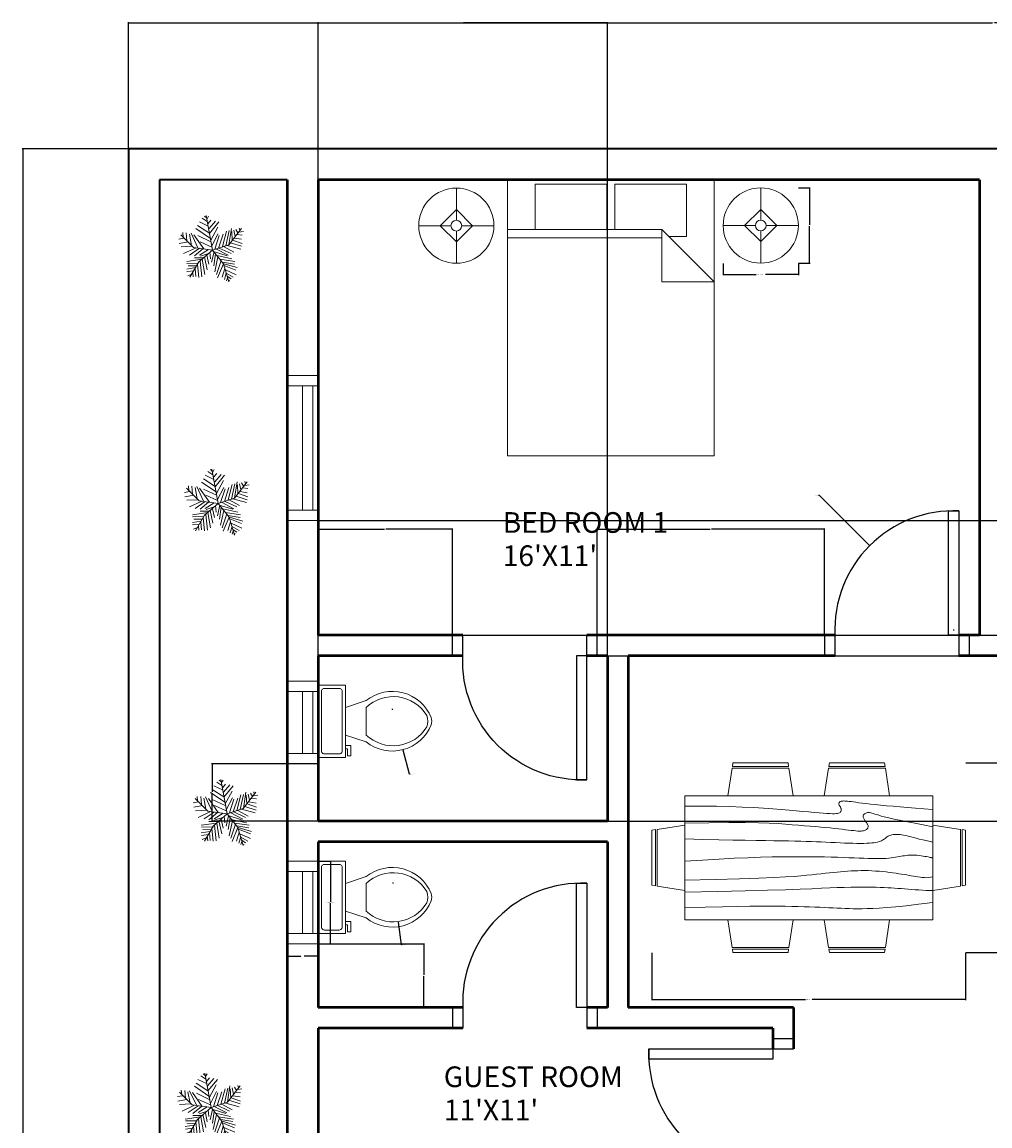
# Model space of a CAD drawing. Units: inches. Extents: x 156 to 720, y 11 to 679.
# Tile 4 of 5: x 156 to 437, y 359 to 679. Entities that reach past the tile are written whole.
import ezdxf

# ---------------------------------------------------------------- set-up
doc = ezdxf.new("R2010")
doc.units = ezdxf.units.IN
for name, color, linetype, lineweight in [('A-ANNO-DIMS', 2, 'Continuous', 18), ('A-AREA-IDEN', 7, 'Continuous', 25), ('A-DOOR', 3, 'Continuous', 25), ('A-FLOR-FIXT', 9, 'Continuous', 18), ('A-FURN', 8, 'Continuous', 18), ('A-GLAZ', 4, 'Continuous', 18), ('A-WALL', 7, 'Continuous', 50), ('C-PROP', 7, 'Continuous', 35), ('E-LITE', 2, 'Continuous', 13), ('L-PLNT', 94, 'Continuous', 13)]:
    doc.layers.add(name, color=color, linetype=linetype, lineweight=lineweight)
doc.styles.get("Standard").update_dxf_attribs({"font": 'arial.ttf'})
doc.dimstyles.get("Standard").update_dxf_attribs({"dimtxt": 0.18, "dimasz": 0.18, "dimexe": 0.18, "dimexo": 0.0625, "dimgap": 0.09, "dimtad": 0, "dimtih": 1, "dimtoh": 1, "dimdec": 4, "dimzin": 0, "dimdsep": 46, "dimtxsty": 'Standard', "dimcen": 0.09, "dimadec": 0, "dimazin": 0, "dimtfac": 1, "dimtdec": 4, "dimtofl": 0, "dimtmove": 0, "dimatfit": 3, "dimfxl": 1, "dimtolj": 1, "dimtzin": 0, "dimarcsym": 0})

# ---------------------------------------------------------------- blocks, each defined once
blk = doc.blocks.new('Bed - Queen')
for p, q in [((0, -80.00003), (0, 0)), ((0, 0), (59.99999, 0)), ((59.99999, 0), (59.99999, -80.00003)), ((7.99999, -1.2), (28.79998, -1.2)), ((7.99999, -14.4), (7.99999, -1.2)), ((28.79998, -1.2), (28.79998, -14.4)), ((31.19999, -1.2), (51.99999, -1.2)), ((31.19999, -14.4), (31.19999, -1.2)), ((51.99999, -1.2), (51.99999, -16.4)), ((0, -14.4), (44.8, -14.4)), ((59.99999, -29.6), (44.8, -14.4)), ((44.8, -14.4), (44.8, -29.6)), ((44.8, -16.8), (0, -16.8)), ((51.99999, -16.4), (46.79936, -16.4)), ((44.8, -29.6), (59.99999, -29.6)), ((59.99999, -80.00003), (0, -80.00003))]:
    blk.add_line(p, q)
blk = doc.blocks.new('Lamp - Table')
for p, q in [((0, 7), (0, 1)), ((0, 3), (-3, 0)), ((3, 0), (0, 3)), ((-1, 0), (-7, 0)), ((-3, 0), (0, -3)), ((0, -3), (3, 0)), ((1, 0), (7, 0)), ((0, -1), (0, -7))]:
    blk.add_line(p, q)
for radius in [7, 1]:
    blk.add_circle((0, 0), radius)
blk = doc.blocks.new('Toilet - top')
for p, q in [((9.5, -6), (9.5, -2)), ((-10, -8.5), (-8, -8.5)), ((-10, -9.5), (-10, -8.5)), ((-7, -9.5), (-10, -9.5)), ((-8, -8.5), (-8, -8)), ((-7, -8), (-7, -9.5)), ((-4, -8), (-6, -14)), ((4, -8), (6, -14)), ((4, -14), (-4, -14))]:
    blk.add_line(p, q)
blk.add_lwpolyline([(10.5, -8), (10.5, 0), (-10.5, 0), (-10.5, -8)], close=True)
for points in [[(-9.5, -2), (-9.5, -6)], [(8.5, -1), (-8.5, -1)], [(-8.5, -7), (8.5, -7)]]:
    blk.add_lwpolyline(points)
for centre, radius, start, end in [((-8.62, -1.88), 0.884, 81.8699, 188.1301), ((8.62, -1.88), 0.884, 351.8699, 98.1301), ((-8.62, -6.12), 0.884, 171.8699, 278.1301), ((8.62, -6.12), 0.884, 261.8699, 8.1301), ((3.52, -21.58), 12.17, 141.4691, 247.9714), ((4.2, -21.82), 11.33, 136.3677, 238.9468), ((-3.52, -21.58), 12.17, 292.0284, 38.5307), ((-4.2, -21.82), 11.33, 301.053, 43.6321), ((0, -27.88), 4, 245.7318, 294.2682), ((0, -29), 4, 254.8605, 285.1395)]:
    blk.add_arc(centre, radius, start, end)
blk = doc.blocks.new('Dining Set - 36 x 72 in.')
for p, q in [((-22.2343, 26.00059), (-23.4847, 17.99762)), ((-22.2304, 26), (-5.7608, 26)), ((-22, 27.5), (-22.1562, 26.50042)), ((-5.8416, 26.5), (-22.1534, 26.5)), ((-22, 27.5), (-6, 27.5)), ((-5.8437, 26.49966), (-6, 27.5)), ((-4.5152, 17.99762), (-5.7655, 25.99926)), ((5.7657, 26.00059), (4.5153, 17.99762)), ((5.7696, 26), (22.2392, 26)), ((6, 27.5), (5.8438, 26.50042)), ((22.1584, 26.5), (5.8466, 26.5)), ((6, 27.5), (22, 27.5)), ((22.1563, 26.49966), (22, 27.5)), ((23.4848, 17.99762), (22.2345, 25.99926)), ((36, 18), (-36, 18)), ((-36, 18), (-36, -18)), ((36, -18), (36, 18)), ((-45.5, 8), (-44.5004, 8.15617)), ((-45.5, 8), (-45.5, -8)), ((-44.5, -8.15843), (-44.5, 8.15338)), ((-44.0006, 8.23428), (-35.9976, 9.48474)), ((-44, 8.23041), (-44, -8.23915)), ((44.0006, 8.23428), (35.9976, 9.48474)), ((44, 8.23041), (44, -8.23915)), ((44.5, -8.15843), (44.5, 8.15338)), ((45.5, 8), (44.5005, 8.15617)), ((45.5, 8), (45.5, -8)), ((-44.4997, -8.15631), (-45.5, -8)), ((-35.9976, -9.48476), (-43.9993, -8.2345)), ((35.9976, -9.48476), (43.9993, -8.2345)), ((44.4997, -8.15631), (45.5, -8)), ((-36, -18), (36, -18)), ((-22.2343, -26.0006), (-23.4847, -17.99762)), ((-4.5152, -17.99762), (-5.7655, -25.99928)), ((5.7657, -26.0006), (4.5153, -17.99762)), ((23.4848, -17.99762), (22.2345, -25.99928)), ((-22.2304, -26), (-5.7608, -26)), ((-22, -27.5), (-22.1562, -26.50044)), ((-5.8416, -26.5), (-22.1534, -26.5)), ((-22, -27.5), (-6, -27.5)), ((-5.8437, -26.49967), (-6, -27.5)), ((5.7696, -26), (22.2392, -26)), ((6, -27.5), (5.8438, -26.50044)), ((22.1584, -26.5), (5.8466, -26.5)), ((6, -27.5), (22, -27.5)), ((22.1563, -26.49967), (22, -27.5))]:
    blk.add_line(p, q)
for points in [[(-36, 15), (-31.1772, 14.97754), (-26.8079, 14.91406), (-22.8538, 14.81543), (-19.276, 14.6875), (-16.0362, 14.53613), (-13.0957, 14.36718), (-10.4159, 14.18652), (-7.9583, 14), (-5.6904, 13.81315), (-3.6035, 13.63021), (-1.6954, 13.45508), (0.0365, 13.29166), (1.5945, 13.14388), (2.9811, 13.01562), (4.1988, 12.9108), (5.25, 12.83333), (6.1393, 12.78613), (6.8802, 12.76823), (7.4883, 12.77767), (7.9792, 12.8125), (8.3685, 12.87077), (8.6719, 12.95052), (8.9049, 13.0498), (9.0833, 13.16666), (9.2205, 13.29899), (9.3216, 13.44401), (9.3895, 13.59879), (9.4271, 13.76041), (9.4373, 13.92594), (9.4232, 14.09245), (9.3875, 14.257), (9.3333, 14.41666), (9.2638, 14.56917), (9.1836, 14.71484), (9.0975, 14.85465), (9.0104, 14.98958), (8.9272, 15.1206), (8.8529, 15.2487), (8.7922, 15.37483), (8.75, 15.5), (8.7305, 15.62467), (8.7344, 15.74739), (8.7617, 15.86621), (8.8125, 15.97916), (8.8867, 16.08431), (8.9844, 16.17968), (9.1055, 16.26334), (9.25, 16.33333), (9.4189, 16.38802), (9.6172, 16.42708), (9.8506, 16.45052), (10.125, 16.45833), (10.4463, 16.45052), (10.8203, 16.42708), (11.2529, 16.38802), (11.75, 16.33333), (12.3184, 16.26318), (12.9694, 16.17838), (13.7151, 16.07991), (14.5677, 15.96875), (15.5395, 15.84586), (16.6426, 15.71224), (17.8893, 15.56884), (19.2917, 15.41666), (20.859, 15.25667), (22.5879, 15.08984), (24.4721, 14.91715), (26.5052, 14.73958), (28.6809, 14.5581), (30.9929, 14.3737), (33.4347, 14.18733), (36, 14)], [(-36, 10), (-28.9766, 10.14274), (-23.1725, 10.20442), (-18.4241, 10.19775), (-14.5677, 10.13541), (-11.4399, 10.03011), (-8.877, 9.89453), (-6.7154, 9.74137), (-4.7917, 9.58333), (-2.9698, 9.43082), (-1.2246, 9.28515), (0.4415, 9.14534), (2.026, 9.01041), (3.5266, 8.87939), (4.9408, 8.7513), (6.266, 8.62516), (7.5, 8.5), (8.6411, 8.37549), (9.6914, 8.2539), (10.6538, 8.13818), (11.5312, 8.03125), (12.3267, 7.93603), (13.043, 7.85547), (13.6831, 7.79248), (14.25, 7.75), (14.7471, 7.7303), (15.1797, 7.73307), (15.5537, 7.75732), (15.875, 7.80208), (16.1494, 7.86637), (16.3828, 7.94922), (16.5811, 8.04964), (16.75, 8.16666), (16.8944, 8.29915), (17.0143, 8.44531), (17.1089, 8.60319), (17.1771, 8.77083), (17.218, 8.94629), (17.2305, 9.1276), (17.2137, 9.31282), (17.1667, 9.5), (17.0895, 9.6875), (16.987, 9.875), (16.8649, 10.0625), (16.7292, 10.25), (16.5856, 10.4375), (16.4401, 10.625), (16.2985, 10.8125), (16.1667, 11), (16.05, 11.18733), (15.9518, 11.3737), (15.8752, 11.5581), (15.8229, 11.73958), (15.798, 11.91715), (15.8034, 12.08984), (15.842, 12.25667), (15.9167, 12.41666), (16.0295, 12.56836), (16.1784, 12.70833), (16.3605, 12.83268), (16.5729, 12.9375), (16.8127, 13.01888), (17.0768, 13.07291), (17.3625, 13.0957), (17.6667, 13.08333), (17.9894, 13.03312), (18.3418, 12.94726), (18.7382, 12.82918), (19.1927, 12.68229), (19.7195, 12.51001), (20.3327, 12.31575), (21.0465, 12.10294), (21.875, 11.875), (22.8357, 11.63354), (23.959, 11.37304), (25.2786, 11.08618), (26.8282, 10.76562), (28.6414, 10.40405), (30.752, 9.99414), (33.1936, 9.52856), (36, 9)], [(-36, 5.5), (-30.7157, 5.3348), (-26.069, 5.20963), (-21.9946, 5.11767), (-18.4271, 5.05208), (-15.3009, 5.00602), (-12.5508, 4.97265), (-10.1112, 4.94515), (-7.9167, 4.91666), (-5.909, 4.88167), (-4.0586, 4.83984), (-2.3429, 4.79215), (-0.7396, 4.73958), (0.7739, 4.6831), (2.22, 4.6237), (3.6213, 4.56233), (5, 4.5), (6.373, 4.43782), (7.7344, 4.3776), (9.0723, 4.32129), (10.375, 4.27083), (11.6309, 4.22819), (12.8281, 4.19531), (13.9551, 4.17415), (15, 4.16666), (15.954, 4.17448), (16.819, 4.19791), (17.6001, 4.23698), (18.3021, 4.29166), (18.9299, 4.36198), (19.4883, 4.44791), (19.9823, 4.54948), (20.4167, 4.66666), (20.7969, 4.79899), (21.1302, 4.94401), (21.4245, 5.09879), (21.6875, 5.26041), (21.9271, 5.42594), (22.1511, 5.59245), (22.3672, 5.757), (22.5834, 5.91666), (22.8065, 6.06868), (23.0404, 6.21093), (23.2879, 6.34147), (23.5521, 6.45833), (23.8358, 6.55957), (24.142, 6.64323), (24.4735, 6.70735), (24.8334, 6.75), (25.2235, 6.76969), (25.642, 6.76692), (26.0858, 6.74267), (26.5521, 6.69791), (27.0379, 6.63362), (27.5404, 6.55078), (28.0565, 6.45036), (28.5834, 6.33333), (29.1242, 6.19987), (29.7071, 6.04687), (30.3661, 5.87044), (31.1354, 5.66666), (32.0493, 5.43164), (33.142, 5.16146), (34.4475, 4.85221), (36, 4.5)], [(-36, -1), (-30.7915, -0.6591), (-26.0195, -0.38216), (-21.6519, -0.16284), (-17.6563, 0.00521), (-14.0005, 0.12833), (-10.6523, 0.21289), (-7.5796, 0.26522), (-4.75, 0.29166), (-2.134, 0.29793), (0.2878, 0.28711), (2.5317, 0.26163), (4.6146, 0.22396), (6.5529, 0.17651), (8.3633, 0.12174), (10.0623, 0.06209), (11.6667, 0), (13.1899, -0.06201), (14.6341, -0.1211), (15.9982, -0.17432), (17.2813, -0.21875), (18.4823, -0.25147), (19.6003, -0.26953), (20.6343, -0.27002), (21.5834, -0.25), (22.4481, -0.20768), (23.2357, -0.14584), (23.9549, -0.06836), (24.6146, 0.02083), (25.2235, 0.11784), (25.7904, 0.21875), (26.3241, 0.31966), (26.8334, 0.41666), (27.3265, 0.50618), (27.8099, 0.58593), (28.2894, 0.65397), (28.7709, 0.70833), (29.2601, 0.74707), (29.763, 0.76823), (30.2855, 0.76985), (30.8334, 0.75), (31.4088, 0.70784), (31.9994, 0.64713), (32.589, 0.57275), (33.1615, 0.48958), (33.7008, 0.4025), (34.1908, 0.3164), (34.6153, 0.23616), (34.9584, 0.16666), (35.2099, 0.11165), (35.3848, 0.07031), (35.504, 0.04069), (35.5886, 0.02083), (35.6594, 0.00879), (35.7377, 0.0026), (35.8442, 0.00032), (36, 0)], [(-36, -6.5), (-27.1843, -6.31267), (-20.084, -6.1263), (-14.469, -5.9419), (-10.1094, -5.76042), (-6.7752, -5.58285), (-4.2363, -5.41016), (-2.2629, -5.24333), (-0.625, -5.08334), (0.8708, -4.93099), (2.2715, -4.78646), (3.5872, -4.64974), (4.8281, -4.52084), (6.0046, -4.39974), (7.127, -4.28646), (8.2053, -4.18099), (9.25, -4.08334), (10.2705, -3.99382), (11.2734, -3.91407), (12.2647, -3.84603), (13.25, -3.79167), (14.2354, -3.75293), (15.2266, -3.73177), (16.2295, -3.73015), (17.25, -3.75), (18.2912, -3.79248), (19.3451, -3.85547), (20.4009, -3.93604), (21.4479, -4.03125), (22.4754, -4.13819), (23.4727, -4.25391), (24.4289, -4.37549), (25.3334, -4.5), (26.1785, -4.62492), (26.9694, -4.74935), (27.7145, -4.87281), (28.4219, -4.99479), (29.1, -5.11483), (29.7572, -5.23242), (30.4016, -5.34709), (31.0417, -5.45834), (31.6837, -5.56437), (32.3262, -5.65821), (32.9658, -5.73153), (33.599, -5.77604), (34.2224, -5.78345), (34.8327, -5.74545), (35.4264, -5.65373), (36, -5.5)], [(-36, -10), (-26.4022, -9.81299), (-18.4675, -9.62891), (-11.9839, -9.45069), (-6.7396, -9.28125), (-2.5226, -9.12354), (0.8789, -8.98047), (3.6769, -8.85498), (6.0833, -8.75), (8.2767, -8.66765), (10.3021, -8.60677), (12.1712, -8.56543), (13.8958, -8.54167), (15.4876, -8.53353), (16.9583, -8.53907), (18.3197, -8.55632), (19.5834, -8.58334), (20.7616, -8.61841), (21.8685, -8.66081), (22.9188, -8.71004), (23.9271, -8.76563), (24.9081, -8.82707), (25.8763, -8.89388), (26.8465, -8.96558), (27.8334, -9.04167), (28.8474, -9.12118), (29.8828, -9.20117), (30.93, -9.27824), (31.9792, -9.34896), (33.0205, -9.40991), (34.0443, -9.45768), (35.0407, -9.48885), (36, -9.5)], [(-36, -14.5), (-30.0881, -14.33513), (-25.0332, -14.21224), (-20.7312, -14.12647), (-17.0781, -14.07292), (-13.97, -14.04671), (-11.3027, -14.04297), (-8.9724, -14.05681), (-6.875, -14.08334), (-4.9224, -14.11833), (-3.0905, -14.16016), (-1.3709, -14.20785), (0.2448, -14.26042), (1.7647, -14.3169), (3.1973, -14.3763), (4.5507, -14.43767), (5.8333, -14.5), (7.0554, -14.5621), (8.235, -14.62175), (9.3922, -14.67652), (10.5469, -14.72396), (11.7192, -14.76164), (12.929, -14.78711), (14.1965, -14.79794), (15.5417, -14.79167), (16.9933, -14.76424), (18.6152, -14.70508), (20.4804, -14.60197), (22.6615, -14.44271), (25.2312, -14.21509), (28.2624, -13.9069), (31.8277, -13.50594), (36, -13)]]:
    blk.add_lwpolyline(points)
blk = doc.blocks.new('*U13')
for p, q in [((-10.186, 53.64), (-13.084, 55.962)), ((0, 0), (-10.5, 57)), ((-9.099, 51.782), (-6.563, 55.962)), ((-5.114, 28.097), (-24.676, 40.636)), ((-7.288, 39.707), (-21.778, 46.673)), ((-8.737, 47.138), (-17.069, 52.711)), ((-7.65, 43.423), (-2.578, 49.46)), ((-5.839, 35.992), (4.667, 48.067)), ((-5.114, 27.632), (10.463, 46.673)), ((-2.941, 16.486), (8.652, 37.85)), ((-47.498, 19.737), (-55.83, 18.344)), ((-31.5, 4.5), (-52.5, 25.5)), ((-48.585, 21.131), (-49.309, 29.026)), ((-43.513, 28.561), (-42.427, 15.558)), ((-38.442, 26.239), (-34.819, 7.663)), ((-35.544, 28.097), (-24.314, 3.947)), ((-14.533, 2.09), (-30.834, 25.31)), ((-3.665, 19.273), (-27.574, 35.527)), ((-24.314, 23.917), (-2.941, 13.7)), ((-1.129, 6.734), (9.014, 26.704)), ((3.942, 1.625), (11.187, 24.381)), ((10.101, 3.483), (17.708, 26.239)), ((16.259, 5.805), (23.142, 31.348)), ((22.055, 7.198), (27.489, 32.277)), ((27, 9), (48, 36)), ((27.127, 9.056), (31.112, 35.992)), ((31.836, 30.883), (32.561, 16.486)), ((35.096, 32.741), (37.27, 22.524)), ((36.183, 19.737), (48.137, 17.88)), ((38.719, 34.134), (41.979, 28.561)), ((40.53, 25.775), (48.862, 24.846)), ((43.791, 29.954), (51.036, 30.883)), ((44.153, 36.456), (45.239, 32.741)), ((-40.615, 13.7), (-55.105, 10.913)), ((-33.37, 6.269), (-52.207, 5.34)), ((-28.299, 3.483), (-47.86, -5.805)), ((-21.416, 3.018), (-38.079, -8.128)), ((0, 0), (-31.5, 4.5)), ((-15.982, 2.09), (-30.11, -9.521)), ((0, 0), (-22.5, -19.5)), ((-6.563, 1.161), (-21.416, -8.128)), ((-20.691, 13.7), (-1.129, 4.876)), ((0, 0), (27, 9)), ((0, 0), (18, -22.5)), ((6.478, 1.625), (26.04, -8.592)), ((11.187, 3.483), (30.749, -5.805)), ((18.07, 5.805), (35.096, -3.483)), ((24.229, 7.663), (46.688, 1.625)), ((29.662, 12.307), (48.137, 6.269)), ((33.285, 16.486), (48.862, 10.913)), ((-17.431, -15.094), (-42.789, -18.809)), ((-15.257, -12.772), (-30.11, -12.772)), ((-6.563, -5.805), (-19.967, -9.985)), ((-17.069, -15.094), (-12.721, -40.172)), ((-13.446, -11.378), (-8.737, -32.741)), ((-9.461, -8.592), (-6.201, -23.453)), ((-4.752, -3.483), (-3.665, -14.629)), ((2.493, -3.019), (-1.491, -20.202)), ((1.769, -2.555), (24.229, -9.521)), ((5.029, -6.27), (2.131, -25.775)), ((9.014, -11.378), (3.58, -35.992)), ((14.085, -16.951), (6.478, -40.172)), ((7.565, -9.056), (32.198, -14.629)), ((12.274, -15.094), (36.907, -18.809)), ((-28.299, -29.026), (-42.789, -31.348)), ((-24.314, -21.596), (-42.427, -22.06)), ((-30.834, -34.135), (-42.427, -35.528)), ((-26.849, -26.24), (-40.253, -25.775)), ((-22.5, -19.5), (-37.5, -45)), ((-29.023, -30.884), (-27.936, -43.887)), ((-25.038, -23.918), (-22.865, -45.281)), ((-20.691, -18.345), (-17.793, -44.352)), ((18.07, -22.524), (8.289, -45.745)), ((20.244, -30.419), (15.897, -44.816)), ((16.259, -19.738), (36.183, -22.989)), ((18, -22.5), (27, -52.5)), ((18.433, -22.524), (40.53, -29.026)), ((19.157, -25.311), (38.719, -33.206)), ((21.331, -32.741), (39.081, -40.636)), ((-34.457, -39.708), (-40.978, -42.494)), ((-32.646, -36.921), (-31.921, -44.352)), ((22.78, -37.85), (19.519, -48.532)), ((22.78, -38.314), (34.372, -44.816)), ((24.591, -45.745), (23.142, -50.854)), ((24.591, -43.423), (30.749, -47.603)), ((26.764, -49.925), (28.213, -50.854))]:
    blk.add_line(p, q)
blk = doc.blocks.new('DOOR-SWING-36IN')
for p, q in [((0, 6), (0, 0)), ((3, 6), (3, 0)), ((39, 6), (39, 0)), ((42, 6), (42, 0))]:
    blk.add_line(p, q)
blk.add_lwpolyline([(39, 6), (36, 6), (36, 42), (39, 42)], close=True)
blk.add_arc((37.5, 7.5), 34.53, 87.5104, 182.4896)
blk = doc.blocks.new('WIN-36IN-WALL9')
for p, q in [((0, 9), (0, 0)), ((39, 9), (3, 9)), ((3, 9), (3, 0)), ((3, 7.5), (39, 7.5)), ((39, 0), (39, 9)), ((42, 0), (42, 9)), ((3, 4.5), (39, 4.5)), ((3, 0), (39, 0))]:
    blk.add_line(p, q)
blk = doc.blocks.new('WIN-18IN-WALL9')
for p, q in [((9, 24), (0, 24)), ((0, 21), (0, 3)), ((9, 21), (0, 21)), ((4.5, 21), (4.5, 3)), ((7.5, 21), (7.5, 3)), ((9, 3), (9, 21)), ((0, 3), (9, 3)), ((0, 0), (9, 0))]:
    blk.add_line(p, q)
blk = doc.blocks.new('*D23')
at = {"layer": 'A-ANNO-DIMS', "color": 0, "lineweight": -2, "transparency": 16777216}
for p, q in [((359.29, 608.96), (359.29, 605.57)), ((381.12, 608.96), (381.12, 605.57)), ((359.47, 605.75), (368.87, 605.75)), ((380.94, 605.75), (371.55, 605.75))]:
    blk.add_line(p, q, dxfattribs=at)
at = {"layer": 'A-ANNO-DIMS', "color": 0, "transparency": 16777216}
for points in [[(359.47, 605.78), (359.47, 605.72), (359.29, 605.75)], [(380.94, 605.78), (380.94, 605.72), (381.12, 605.75)]]:
    blk.add_solid(points, dxfattribs=at)
at = {"layer": 'Defpoints', "color": 0, "transparency": 16777216}
for p in [(359.29, 609.02), (381.12, 609.02), (381.12, 605.75)]:
    blk.add_point(p, dxfattribs=at)
at = {"layer": 'A-ANNO-DIMS', "color": 0, "transparency": 16777216, "insert": (370.21, 605.75), "char_height": 0.18, "attachment_point": 5}
blk.add_mtext('\\A1;TABLE LAMP 22 TYP.', dxfattribs=at)
blk = doc.blocks.new('*D24')
at = {"layer": 'A-ANNO-DIMS', "color": 0, "lineweight": -2, "transparency": 16777216}
for p, q in [((381.18, 630.84), (384.57, 630.84)), ((384.39, 630.66), (384.39, 620.11)), ((384.39, 609.2), (384.39, 619.75)), ((381.18, 609.02), (384.57, 609.02))]:
    blk.add_line(p, q, dxfattribs=at)
at = {"layer": 'A-ANNO-DIMS', "color": 0, "transparency": 16777216}
for points in [[(384.36, 630.66), (384.42, 630.66), (384.39, 630.84)], [(384.36, 609.2), (384.42, 609.2), (384.39, 609.02)]]:
    blk.add_solid(points, dxfattribs=at)
at = {"layer": 'Defpoints', "color": 0, "transparency": 16777216}
for p in [(381.12, 630.84), (384.39, 630.84), (381.12, 609.02)]:
    blk.add_point(p, dxfattribs=at)
at = {"layer": 'A-ANNO-DIMS', "color": 0, "transparency": 16777216, "insert": (384.39, 619.93), "char_height": 0.18, "attachment_point": 5}
blk.add_mtext('\\A1;22 TYP.', dxfattribs=at)
blk = doc.blocks.new('*D31')
at = {"layer": 'A-ANNO-DIMS', "color": 0, "lineweight": -2, "transparency": 16777216}
for p, q in [((241.79, 435.59), (245.5, 435.59)), ((245.32, 435.41), (245.32, 423.77)), ((245.32, 411.77), (245.32, 423.41)), ((241.79, 411.59), (245.5, 411.59))]:
    blk.add_line(p, q, dxfattribs=at)
at = {"layer": 'A-ANNO-DIMS', "color": 0, "transparency": 16777216}
for points in [[(245.29, 435.41), (245.35, 435.41), (245.32, 435.59)], [(245.29, 411.77), (245.35, 411.77), (245.32, 411.59)]]:
    blk.add_solid(points, dxfattribs=at)
at = {"layer": 'Defpoints', "color": 0, "transparency": 16777216}
for p in [(241.72, 435.59), (245.32, 435.59), (241.72, 411.59)]:
    blk.add_point(p, dxfattribs=at)
at = {"layer": 'A-ANNO-DIMS', "color": 0, "transparency": 16777216, "insert": (245.32, 423.59), "char_height": 0.18, "attachment_point": 5}
blk.add_mtext('\\A1;WINDOW B 24 TYP.', dxfattribs=at)
blk = doc.blocks.new('*D32')
at = {"layer": 'A-ANNO-DIMS', "color": 0, "lineweight": -2, "transparency": 16777216}
for p, q in [((232.72, 411.53), (232.72, 407.81)), ((241.72, 411.53), (241.72, 407.81)), ((232.9, 407.99), (236.77, 407.99)), ((241.54, 407.99), (237.68, 407.99))]:
    blk.add_line(p, q, dxfattribs=at)
at = {"layer": 'A-ANNO-DIMS', "color": 0, "transparency": 16777216}
for points in [[(232.9, 408.02), (232.9, 407.96), (232.72, 407.99)], [(241.54, 408.02), (241.54, 407.96), (241.72, 407.99)]]:
    blk.add_solid(points, dxfattribs=at)
at = {"layer": 'Defpoints', "color": 0, "transparency": 16777216}
for p in [(232.72, 411.59), (241.72, 411.59), (241.72, 407.99)]:
    blk.add_point(p, dxfattribs=at)
at = {"layer": 'A-ANNO-DIMS', "color": 0, "transparency": 16777216, "insert": (237.22, 407.99), "char_height": 0.18, "attachment_point": 5}
blk.add_mtext('\\A1;9 TYP.', dxfattribs=at)
blk = doc.blocks.new('*D41')
at = {"layer": 'A-ANNO-DIMS', "color": 0, "lineweight": -2, "transparency": 16777216}
for p, q in [((338.64, 408.99), (338.64, 395.23)), ((429.64, 408.99), (429.64, 395.23)), ((338.82, 395.41), (383.18, 395.41)), ((429.46, 395.41), (385.09, 395.41))]:
    blk.add_line(p, q, dxfattribs=at)
at = {"layer": 'A-ANNO-DIMS', "color": 0, "transparency": 16777216}
for points in [[(338.82, 395.44), (338.82, 395.38), (338.64, 395.41)], [(429.46, 395.44), (429.46, 395.38), (429.64, 395.41)]]:
    blk.add_solid(points, dxfattribs=at)
at = {"layer": 'Defpoints', "color": 0, "transparency": 16777216}
for p in [(338.64, 409.06), (429.64, 409.06), (429.64, 395.41)]:
    blk.add_point(p, dxfattribs=at)
at = {"layer": 'A-ANNO-DIMS', "color": 0, "transparency": 16777216, "insert": (384.14, 395.41), "char_height": 0.18, "attachment_point": 5}
blk.add_mtext('\\A1;DINING SET 91', dxfattribs=at)
blk = doc.blocks.new('*D42')
at = {"layer": 'A-ANNO-DIMS', "color": 0, "lineweight": -2, "transparency": 16777216}
for p, q in [((429.7, 464.06), (443.47, 464.06)), ((443.29, 463.88), (443.29, 436.74)), ((443.29, 409.24), (443.29, 436.37)), ((429.7, 409.06), (443.47, 409.06))]:
    blk.add_line(p, q, dxfattribs=at)
at = {"layer": 'A-ANNO-DIMS', "color": 0, "transparency": 16777216}
for points in [[(443.26, 463.88), (443.32, 463.88), (443.29, 464.06)], [(443.26, 409.24), (443.32, 409.24), (443.29, 409.06)]]:
    blk.add_solid(points, dxfattribs=at)
at = {"layer": 'Defpoints', "color": 0, "transparency": 16777216}
for p in [(429.64, 464.06), (443.29, 464.06), (429.64, 409.06)]:
    blk.add_point(p, dxfattribs=at)
at = {"layer": 'A-ANNO-DIMS', "color": 0, "transparency": 16777216, "insert": (443.29, 436.56), "char_height": 0.18, "attachment_point": 5}
blk.add_mtext('\\A1;55', dxfattribs=at)
blk = doc.blocks.new('*D49')
at = {"layer": 'A-ANNO-DIMS', "color": 0, "lineweight": -2, "transparency": 16777216}
for p, q in [((186.72, 642.21), (186.72, 678.94)), ((688.72, 642.21), (688.72, 678.94)), ((186.9, 678.76), (437.44, 678.76)), ((688.54, 678.76), (438.01, 678.76))]:
    blk.add_line(p, q, dxfattribs=at)
at = {"layer": 'A-ANNO-DIMS', "color": 0, "transparency": 16777216}
for points in [[(186.9, 678.79), (186.9, 678.73), (186.72, 678.76)], [(688.54, 678.79), (688.54, 678.73), (688.72, 678.76)]]:
    blk.add_solid(points, dxfattribs=at)
at = {"layer": 'Defpoints', "color": 0, "transparency": 16777216}
for p in [(688.72, 678.76), (186.72, 642.15), (688.72, 642.15)]:
    blk.add_point(p, dxfattribs=at)
at = {"layer": 'A-ANNO-DIMS', "color": 0, "transparency": 16777216, "insert": (437.72, 678.76), "char_height": 0.18, "attachment_point": 5}
blk.add_mtext('\\A1;502', dxfattribs=at)
blk = doc.blocks.new('*D50')
at = {"layer": 'A-ANNO-DIMS', "color": 0, "lineweight": -2, "transparency": 16777216}
for p, q in [((186.66, 642.15), (155.84, 642.15)), ((156.02, 641.97), (156.02, 342.33)), ((156.02, 42.33), (156.02, 341.97)), ((186.66, 42.15), (155.84, 42.15))]:
    blk.add_line(p, q, dxfattribs=at)
at = {"layer": 'A-ANNO-DIMS', "color": 0, "transparency": 16777216}
for points in [[(155.99, 641.97), (156.05, 641.97), (156.02, 642.15)], [(155.99, 42.33), (156.05, 42.33), (156.02, 42.15)]]:
    blk.add_solid(points, dxfattribs=at)
at = {"layer": 'Defpoints', "color": 0, "transparency": 16777216}
for p in [(156.02, 642.15), (186.72, 642.15), (186.72, 42.15)]:
    blk.add_point(p, dxfattribs=at)
at = {"layer": 'A-ANNO-DIMS', "color": 0, "transparency": 16777216, "insert": (156.02, 342.15), "char_height": 0.18, "attachment_point": 5}
blk.add_mtext('\\A1;600', dxfattribs=at)
blk = doc.blocks.new('*D66')
at = {"layer": 'A-ANNO-DIMS', "color": 0, "lineweight": -2, "transparency": 16777216}
for p, q in [((241.72, 447.21), (241.72, 678.94)), ((325.72, 447.21), (325.72, 678.94)), ((241.9, 678.76), (283.5, 678.76)), ((325.54, 678.76), (283.94, 678.76))]:
    blk.add_line(p, q, dxfattribs=at)
at = {"layer": 'A-ANNO-DIMS', "color": 0, "transparency": 16777216}
for points in [[(241.9, 678.79), (241.9, 678.73), (241.72, 678.76)], [(325.54, 678.79), (325.54, 678.73), (325.72, 678.76)]]:
    blk.add_solid(points, dxfattribs=at)
at = {"layer": 'Defpoints', "color": 0, "transparency": 16777216}
for p in [(325.72, 678.76), (241.72, 447.15), (325.72, 447.15)]:
    blk.add_point(p, dxfattribs=at)
at = {"layer": 'A-ANNO-DIMS', "color": 0, "transparency": 16777216, "insert": (283.72, 678.76), "char_height": 0.18, "attachment_point": 5}
blk.add_mtext('\\A1;84', dxfattribs=at)
blk = doc.blocks.new('*D67')
at = {"layer": 'A-ANNO-DIMS', "color": 0, "lineweight": -2, "transparency": 16777216}
for p, q in [((325.79, 495.15), (719.6, 495.15)), ((719.42, 494.97), (719.42, 471.33)), ((719.42, 447.33), (719.42, 470.97)), ((325.79, 447.15), (719.6, 447.15))]:
    blk.add_line(p, q, dxfattribs=at)
at = {"layer": 'A-ANNO-DIMS', "color": 0, "transparency": 16777216}
for points in [[(719.39, 494.97), (719.45, 494.97), (719.42, 495.15)], [(719.39, 447.33), (719.45, 447.33), (719.42, 447.15)]]:
    blk.add_solid(points, dxfattribs=at)
at = {"layer": 'Defpoints', "color": 0, "transparency": 16777216}
for p in [(325.72, 495.15), (719.42, 495.15), (325.72, 447.15)]:
    blk.add_point(p, dxfattribs=at)
at = {"layer": 'A-ANNO-DIMS', "color": 0, "transparency": 16777216, "insert": (719.42, 471.15), "char_height": 0.18, "attachment_point": 5}
blk.add_mtext('\\A1;48', dxfattribs=at)
blk = doc.blocks.new('*D70')
at = {"layer": 'A-ANNO-DIMS', "color": 0, "lineweight": -2, "transparency": 16777216}
for p, q in [((241.72, 501.21), (241.72, 532.03)), ((241.9, 531.85), (261, 531.85)), ((280.54, 531.85), (261.44, 531.85)), ((280.72, 501.21), (280.72, 532.03))]:
    blk.add_line(p, q, dxfattribs=at)
at = {"layer": 'A-ANNO-DIMS', "color": 0, "transparency": 16777216}
for points in [[(241.9, 531.88), (241.9, 531.82), (241.72, 531.85)], [(280.54, 531.88), (280.54, 531.82), (280.72, 531.85)]]:
    blk.add_solid(points, dxfattribs=at)
at = {"layer": 'Defpoints', "color": 0, "transparency": 16777216}
for p in [(280.72, 531.85), (241.72, 501.15), (280.72, 501.15)]:
    blk.add_point(p, dxfattribs=at)
at = {"layer": 'A-ANNO-DIMS', "color": 0, "transparency": 16777216, "insert": (261.22, 531.85), "char_height": 0.18, "attachment_point": 5}
blk.add_mtext('\\A1;39', dxfattribs=at)
blk = doc.blocks.new('*D71')
at = {"layer": 'A-ANNO-DIMS', "color": 0, "lineweight": -2, "transparency": 16777216}
for p, q in [((322.72, 501.21), (322.72, 532.03)), ((322.9, 531.85), (355.5, 531.85)), ((388.54, 531.85), (355.94, 531.85)), ((388.72, 501.21), (388.72, 532.03))]:
    blk.add_line(p, q, dxfattribs=at)
at = {"layer": 'A-ANNO-DIMS', "color": 0, "transparency": 16777216}
for points in [[(322.9, 531.88), (322.9, 531.82), (322.72, 531.85)], [(388.54, 531.88), (388.54, 531.82), (388.72, 531.85)]]:
    blk.add_solid(points, dxfattribs=at)
at = {"layer": 'Defpoints', "color": 0, "transparency": 16777216}
for p in [(388.72, 531.85), (322.72, 501.15), (388.72, 501.15)]:
    blk.add_point(p, dxfattribs=at)
at = {"layer": 'A-ANNO-DIMS', "color": 0, "transparency": 16777216, "insert": (355.72, 531.85), "char_height": 0.18, "attachment_point": 5}
blk.add_mtext('\\A1;66', dxfattribs=at)
blk = doc.blocks.new('*D72')
at = {"layer": 'A-ANNO-DIMS', "color": 0, "lineweight": -2, "transparency": 16777216}
for p, q in [((241.79, 534.4), (719.6, 534.4)), ((719.42, 534.22), (719.42, 517.96)), ((719.42, 501.33), (719.42, 517.59)), ((241.79, 501.15), (719.6, 501.15))]:
    blk.add_line(p, q, dxfattribs=at)
at = {"layer": 'A-ANNO-DIMS', "color": 0, "transparency": 16777216}
for points in [[(719.39, 534.22), (719.45, 534.22), (719.42, 534.4)], [(719.39, 501.33), (719.45, 501.33), (719.42, 501.15)]]:
    blk.add_solid(points, dxfattribs=at)
at = {"layer": 'Defpoints', "color": 0, "transparency": 16777216}
for p in [(241.72, 534.4), (719.42, 534.4), (241.72, 501.15)]:
    blk.add_point(p, dxfattribs=at)
at = {"layer": 'A-ANNO-DIMS', "color": 0, "transparency": 16777216, "insert": (719.42, 517.78), "char_height": 0.18, "attachment_point": 5}
blk.add_mtext('\\A1;33.25', dxfattribs=at)
blk = doc.blocks.new('*D75')
at = {"layer": 'A-ANNO-DIMS', "color": 0, "lineweight": -2, "transparency": 16777216}
for p, q in [((241.79, 411.59), (272.6, 411.59)), ((272.42, 411.41), (272.42, 402.55)), ((272.42, 393.33), (272.42, 402.19)), ((241.79, 393.15), (272.6, 393.15))]:
    blk.add_line(p, q, dxfattribs=at)
at = {"layer": 'A-ANNO-DIMS', "color": 0, "transparency": 16777216}
for points in [[(272.39, 411.41), (272.45, 411.41), (272.42, 411.59)], [(272.39, 393.33), (272.45, 393.33), (272.42, 393.15)]]:
    blk.add_solid(points, dxfattribs=at)
at = {"layer": 'Defpoints', "color": 0, "transparency": 16777216}
for p in [(241.72, 411.59), (241.72, 393.15), (272.42, 393.15)]:
    blk.add_point(p, dxfattribs=at)
at = {"layer": 'A-ANNO-DIMS', "color": 0, "transparency": 16777216, "insert": (272.42, 402.37), "char_height": 0.18, "attachment_point": 5}
blk.add_mtext('\\A1;18.44', dxfattribs=at)
blk = doc.blocks.new('*D76')
at = {"layer": 'A-ANNO-DIMS', "color": 0, "lineweight": -2, "transparency": 16777216}
for p, q in [((241.66, 463.78), (210.84, 463.78)), ((211.02, 463.6), (211.02, 455.65)), ((211.02, 447.33), (211.02, 455.29)), ((241.66, 447.15), (210.84, 447.15))]:
    blk.add_line(p, q, dxfattribs=at)
at = {"layer": 'A-ANNO-DIMS', "color": 0, "transparency": 16777216}
for points in [[(210.99, 463.6), (211.05, 463.6), (211.02, 463.78)], [(210.99, 447.33), (211.05, 447.33), (211.02, 447.15)]]:
    blk.add_solid(points, dxfattribs=at)
at = {"layer": 'Defpoints', "color": 0, "transparency": 16777216}
for p in [(211.02, 463.78), (241.72, 463.78), (241.72, 447.15)]:
    blk.add_point(p, dxfattribs=at)
at = {"layer": 'A-ANNO-DIMS', "color": 0, "transparency": 16777216, "insert": (211.02, 455.47), "char_height": 0.18, "attachment_point": 5}
blk.add_mtext('\\A1;16.63', dxfattribs=at)
blk = doc.blocks.new('*D80')
at = {"layer": 'A-ANNO-DIMS', "color": 0, "lineweight": -2, "transparency": 16777216}
for p, q in [((386.97, 541.72), (387.15, 541.72)), ((387.15, 541.72), (401.68, 527.2)), ((426.22, 502.56), (426.22, 502.74)), ((426.13, 502.65), (426.31, 502.65))]:
    blk.add_line(p, q, dxfattribs=at)
at = {"layer": 'A-ANNO-DIMS', "color": 0, "transparency": 16777216}
blk.add_solid([(401.7, 527.22), (401.66, 527.18), (401.81, 527.07)], dxfattribs=at)
at = {"layer": 'Defpoints', "color": 0, "transparency": 16777216}
for p in [(401.81, 527.07), (426.22, 502.65)]:
    blk.add_point(p, dxfattribs=at)
at = {"layer": 'A-ANNO-DIMS', "color": 0, "transparency": 16777216, "insert": (386.3, 541.72), "char_height": 0.18, "attachment_point": 5}
blk.add_mtext('\\A1;4X R34.53', dxfattribs=at)
blk = doc.blocks.new('*D85')
at = {"layer": 'A-ANNO-DIMS', "color": 0, "lineweight": -2, "transparency": 16777216}
for p, q in [((263.21, 479.67), (263.39, 479.67)), ((263.3, 479.58), (263.3, 479.76)), ((268.25, 460.84), (266.44, 467.73)), ((268.43, 460.84), (268.25, 460.84))]:
    blk.add_line(p, q, dxfattribs=at)
at = {"layer": 'A-ANNO-DIMS', "color": 0, "transparency": 16777216}
blk.add_solid([(266.47, 467.73), (266.41, 467.72), (266.4, 467.9)], dxfattribs=at)
at = {"layer": 'Defpoints', "color": 0, "transparency": 16777216}
for p in [(263.3, 479.67), (266.4, 467.9)]:
    blk.add_point(p, dxfattribs=at)
at = {"layer": 'A-ANNO-DIMS', "color": 0, "transparency": 16777216, "insert": (269.1, 460.84), "char_height": 0.18, "attachment_point": 5}
blk.add_mtext('\\A1;6X R12.17', dxfattribs=at)
blk = doc.blocks.new('*D86')
at = {"layer": 'A-ANNO-DIMS', "color": 0, "lineweight": -2, "transparency": 16777216}
for p, q in [((263.45, 429.29), (263.63, 429.29)), ((263.54, 429.2), (263.54, 429.38)), ((265.96, 411.33), (265.08, 417.88)), ((266.14, 411.33), (265.96, 411.33))]:
    blk.add_line(p, q, dxfattribs=at)
at = {"layer": 'A-ANNO-DIMS', "color": 0, "transparency": 16777216}
blk.add_solid([(265.1, 417.89), (265.05, 417.88), (265.05, 418.06)], dxfattribs=at)
at = {"layer": 'Defpoints', "color": 0, "transparency": 16777216}
for p in [(263.54, 429.29), (265.05, 418.06)]:
    blk.add_point(p, dxfattribs=at)
at = {"layer": 'A-ANNO-DIMS', "color": 0, "transparency": 16777216, "insert": (266.81, 411.33), "char_height": 0.18, "attachment_point": 5}
blk.add_mtext('\\A1;6X R11.33', dxfattribs=at)

msp = doc.modelspace()

# ---------------------------------------------------------------- linework, layer by layer
at = {"layer": 'A-WALL'}
for p, q in [((232.7236, 633.1514), (232.7236, 246.1514)), ((241.7236, 633.1514), (241.7236, 501.1514)), ((433.7236, 633.1514), (241.7236, 633.1514)), ((433.7236, 633.1514), (433.7236, 501.1514)), ((283.7236, 501.1514), (241.7236, 501.1514)), ((391.7236, 501.1514), (319.7236, 501.1514)), ((433.7236, 501.1514), (427.7236, 501.1514)), ((241.7236, 495.1514), (241.7236, 447.1514)), ((283.7236, 495.1514), (241.7236, 495.1514)), ((325.7236, 495.1514), (319.7236, 495.1514)), ((325.7236, 495.1514), (325.7236, 447.1514)), ((331.7236, 495.1514), (331.7236, 393.1514)), ((391.7236, 495.1514), (331.7236, 495.1514)), ((445.7236, 495.1514), (427.7236, 495.1514)), ((325.7236, 447.1514), (241.7236, 447.1514)), ((325.7236, 441.1514), (241.7236, 441.1514)), ((241.7236, 441.1514), (241.7236, 393.1514)), ((325.7236, 441.1514), (325.7236, 393.1514)), ((283.7236, 393.1514), (241.7236, 393.1514)), ((325.7236, 393.1514), (319.7236, 393.1514)), ((379.7236, 393.1514), (331.7236, 393.1514)), ((379.7236, 393.1514), (379.7236, 381.1514)), ((241.7236, 387.1514), (241.7236, 255.1514)), ((283.7236, 387.1514), (241.7236, 387.1514)), ((373.7236, 387.1514), (319.7236, 387.1514)), ((373.7236, 387.1514), (373.7236, 381.1514))]:
    msp.add_line(p, q, dxfattribs=at)
at = {"layer": 'C-PROP'}
for p, q in [((688.7236, 642.1514), (186.7236, 642.1514)), ((186.7236, 642.1514), (186.7236, 51.1514)), ((195.7236, 633.1514), (195.7236, 51.1514)), ((232.7236, 633.1514), (195.7236, 633.1514))]:
    msp.add_line(p, q, dxfattribs=at)

# ---------------------------------------------------------------- block references
at = {"layer": 'A-DOOR'}
for p in [(388.724, 495.151), (280.724, 387.151)]:
    msp.add_blockref('DOOR-SWING-36IN', p, dxfattribs=at)
at = {"layer": 'A-DOOR', "extrusion": (0, 0, -1), "zscale": -1, "rotation": 180}
msp.add_blockref('DOOR-SWING-36IN', (-280.724, 501.1518), dxfattribs=at)
at = {"layer": 'A-DOOR', "rotation": 89.99999999999989}
msp.add_blockref('DOOR-SWING-36IN', (379.724, 342.1518), dxfattribs=at)
at = {"layer": 'A-FLOR-FIXT', "rotation": 90}
for p in [(241.7236, 476.1505), (241.7236, 425.0911)]:
    msp.add_blockref('Toilet - top', p, dxfattribs=at)
at = {"layer": 'A-FURN'}
for name, p in [('Bed - Queen', (296.698, 633.1496)), ('Dining Set - 36 x 72 in.', (384.1356, 436.556))]:
    msp.add_blockref(name, p, dxfattribs=at)
at = {"layer": 'A-GLAZ', "rotation": 270.0000000000003}
msp.add_blockref('WIN-36IN-WALL9', (232.7232, 576.402), dxfattribs=at)
at = {"layer": 'A-GLAZ'}
for p in [(232.724, 463.783), (232.724, 411.591)]:
    msp.add_blockref('WIN-18IN-WALL9', p, dxfattribs=at)
at = {"layer": 'E-LITE', "xscale": 1.558829175044203, "yscale": 1.558829175044203, "zscale": 1.558829175044203}
for p in [(281.8596, 619.8835), (370.2061, 619.9318)]:
    msp.add_blockref('Lamp - Table', p, dxfattribs=at)
at = {"layer": 'L-PLNT', "xscale": 0.175286236255467, "yscale": 0.175286236255467, "zscale": 0.175286236255467}
for p in [(211.1043, 612.7979), (212.7571, 539.3084), (215.3002, 449.2618), (210.6733, 364.0639)]:
    msp.add_blockref('*U13', p, dxfattribs=at)

# ---------------------------------------------------------------- texts
at = {"layer": 'A-AREA-IDEN'}
for s, p in [('BED ROOM 1', (295.3167, 530.7947)), ("16'X11'", (295.3167, 521.1562)), ('GUEST ROOM', (278.21, 370.0171)), ("11'X11'", (278.21, 360.3786))]:
    msp.add_text(s, height=6, dxfattribs=at).set_placement(p)

# ---------------------------------------------------------------- dimensions: what is measured, and where the dimension line sits
at = {"layer": 'A-ANNO-DIMS'}
for base, p1, p2, picture, middle in [((688.7236, 678.7597), (186.7236, 642.1514), (688.7236, 642.1514), '*D49', (437.7236, 678.7597)), ((325.7236, 678.7597), (241.7236, 447.1514), (325.7236, 447.1514), '*D66', (283.7236, 678.7597)), ((388.7236, 531.8514), (322.7236, 501.1514), (388.7236, 501.1514), '*D71', (355.7236, 531.8514))]:
    dim = msp.add_linear_dim(base=base, p1=p1, p2=p2, dimstyle='Standard', override={"dimdec": 0, "dimlfac": 1, "dimrnd": 0, "dimzin": 0, "dimdsep": 46, "dimlunit": 2}, dxfattribs=at)
    dim.commit()
    dim.dimension.update_dxf_attribs({"geometry": picture, "text_midpoint": middle})
for base, p1, p2, angle, override, picture, middle in [((156.0236, 642.1514), (186.7236, 42.1514), (186.7236, 642.1514), 90, {"dimdec": 0, "dimlfac": 1, "dimrnd": 0, "dimzin": 0, "dimdsep": 46, "dimlunit": 2}, '*D50', (156.0236, 342.1514)), ((719.4236, 534.4018), (241.7236, 501.1514), (241.7236, 534.4018), 90, {"dimdec": 2, "dimlfac": 1, "dimrnd": 0, "dimzin": 0, "dimdsep": 46, "dimlunit": 2}, '*D72', (719.4236, 517.7766)), ((280.7236, 531.8514), (241.7236, 501.1514), (280.7236, 501.1514), 0, {"dimdec": 0, "dimlfac": 1, "dimrnd": 0, "dimzin": 0, "dimdsep": 46, "dimlunit": 2}, '*D70', (261.2236, 531.8514)), ((719.4236, 495.1514), (325.7236, 447.1514), (325.7236, 495.1514), 90, {"dimdec": 0, "dimlfac": 1, "dimrnd": 0, "dimzin": 0, "dimdsep": 46, "dimlunit": 2}, '*D67', (719.4236, 471.1514)), ((211.0236, 463.783), (241.7236, 447.1514), (241.7236, 463.783), 90, {"dimdec": 2, "dimlfac": 1, "dimrnd": 0, "dimzin": 0, "dimdsep": 46, "dimlunit": 2}, '*D76', (211.0236, 455.4672)), ((443.2856, 464.056), (429.6356, 409.056), (429.6356, 464.056), 90, {"dimdec": 0, "dimlfac": 1, "dimrnd": 0, "dimzin": 0, "dimdsep": 46, "dimlunit": 2}, '*D42', (443.2856, 436.556)), ((272.4236, 393.1514), (241.7236, 411.5911), (241.7236, 393.1514), 270, {"dimdec": 2, "dimlfac": 1, "dimrnd": 0, "dimzin": 0, "dimdsep": 46, "dimlunit": 2}, '*D75', (272.4236, 402.3712))]:
    dim = msp.add_linear_dim(base=base, p1=p1, p2=p2, angle=angle, dimstyle='Standard', override=override, dxfattribs=at)
    dim.commit()
    dim.dimension.update_dxf_attribs({"geometry": picture, "text_midpoint": middle})
for base, p1, p2, text, picture, middle in [((384.3915, 630.8436), (381.1179, 609.02), (381.1179, 630.8436), '<> TYP.', '*D24', (384.3915, 619.9318)), ((245.3236, 435.5911), (241.7236, 411.5911), (241.7236, 435.5911), 'WINDOW B <> TYP.', '*D31', (245.3236, 423.5911))]:
    dim = msp.add_linear_dim(base=base, p1=p1, p2=p2, angle=90, text=text, dimstyle='Standard', override={"dimdec": 0, "dimlfac": 1, "dimrnd": 0, "dimzin": 0, "dimdsep": 46, "dimlunit": 2}, dxfattribs=at)
    dim.commit()
    dim.dimension.update_dxf_attribs({"geometry": picture, "text_midpoint": middle})
for base, p1, p2, text, picture, middle in [((381.1179, 605.7465), (359.2943, 609.02), (381.1179, 609.02), 'TABLE LAMP <> TYP.', '*D23', (370.2061, 605.7465)), ((241.7236, 407.9911), (232.7236, 411.5911), (241.7236, 411.5911), '<> TYP.', '*D32', (237.2236, 407.9911)), ((429.6356, 395.406), (338.6356, 409.056), (429.6356, 409.056), 'DINING SET <>', '*D41', (384.1356, 395.406))]:
    dim = msp.add_linear_dim(base=base, p1=p1, p2=p2, text=text, dimstyle='Standard', override={"dimdec": 0, "dimlfac": 1, "dimrnd": 0, "dimzin": 0, "dimdsep": 46, "dimlunit": 2}, dxfattribs=at)
    dim.commit()
    dim.dimension.update_dxf_attribs({"geometry": picture, "text_midpoint": middle})
for center, mpoint, text, picture, middle in [((426.2236, 502.6514), (401.8054, 527.0696), '4X <>', '*D80', (386.2976, 541.7206)), ((263.3041, 479.6701), (266.3959, 467.9004), '6X <>', '*D85', (269.1047, 460.8386)), ((263.541, 429.291), (265.051, 418.0629), '6X <>', '*D86', (266.8107, 411.3261))]:
    dim = msp.add_radius_dim(center=center, mpoint=mpoint, text=text, dimstyle='Standard', override={"dimdec": 2, "dimlfac": 1, "dimrnd": 0, "dimzin": 0, "dimdsep": 46, "dimlunit": 2}, dxfattribs=at)
    dim.commit()
    dim.dimension.update_dxf_attribs({"geometry": picture, "text_midpoint": middle, "dimtype": 164})

doc.saveas('drawing.dxf')
